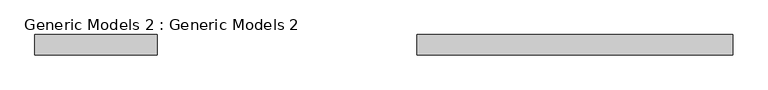
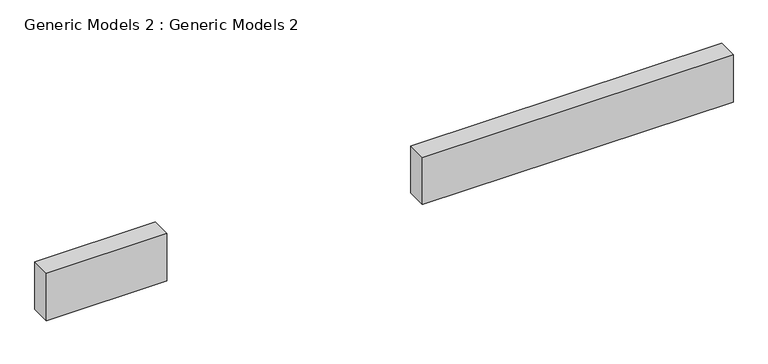
"""IFC4 building model written with IfcOpenShell, lengths in millimetres: proxy geometry, Generic Models 2 : Generic Models 2."""

from ifc_helpers import new_model, si_unit, frame, origin, place, context, project, spatial, polyline, outline, extrude, source, transform, mapped, element, save


def generic_models_2_generic_models_2_082925ae(model_context):
    return source(origin(), model_context, "Body", "SweptSolid", [
        extrude(outline(polyline([(4631.2084916, -8759.0599223), (-93.1915084, -8759.0599223), (-93.1915084, -8454.2599223), (4631.2084916, -8454.2599223), (4631.2084916, -8759.0599223)])), frame((0.0, 0.0, 312.5414352), z_axis=(0.0, 0.0, 1.0), x_axis=(1.0, 0.0, 0.0)), (0.0, 0.0, 1.0), 762.0),
        extrude(outline(polyline([(-3980.8650513, -8759.0599223), (-5809.6650513, -8759.0599223), (-5809.6650513, -8454.2599223), (-3980.8650513, -8454.2599223), (-3980.8650513, -8759.0599223)])), frame((0.0, 0.0, 444.9112051), z_axis=(0.0, 0.0, 1.0), x_axis=(1.0, 0.0, 0.0)), (0.0, 0.0, 1.0), 762.0),
    ])


if __name__ == "__main__":
    model = new_model("IFC4")
    model_context = context("Model", 3, world=origin())
    ifc_project = project(units=[si_unit("LENGTHUNIT", "METRE", prefix="MILLI")], contexts=[model_context])
    site = spatial("IfcSite", under=ifc_project)
    building = spatial("IfcBuilding", under=site)
    placement = place(None, origin())
    generic_models_2_generic_models_2_shape = generic_models_2_generic_models_2_082925ae(model_context)
    element("IfcBuildingElementProxy", 1, Name="Generic Models 2 : Generic Models 2", ObjectType="Generic Models 2 : Generic Models 2", at=placement, inside=building, context=model_context, shape_type="MappedRepresentation", body=[
        mapped(generic_models_2_generic_models_2_shape, transform((0.0, 0.0, 0.0), x_axis=(1.0, 0.0, 0.0), y_axis=(0.0, 1.0, 0.0), z_axis=(0.0, 0.0, 1.0))),
    ])
    save(model, "model.ifc")

# Revit data of these elements
# Element 1 (IfcBuildingElementProxy, "Generic Models 2 : Generic Models 2")
#   Materials on its faces: "Carpet (1)"
# Materials
#   "Carpet (1)": class "Carpet", colour RGB 124 80 67, transparency 0, Description = "Interior finish", Cost = 0
